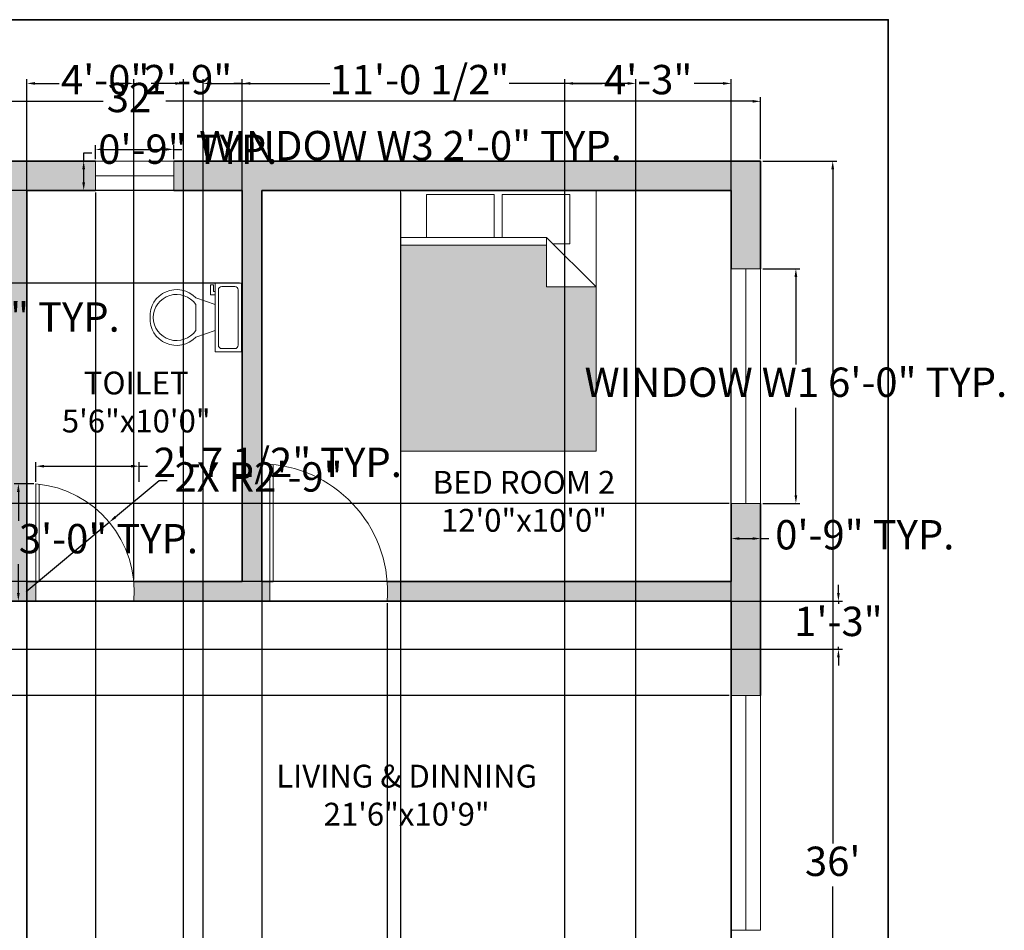
# Model space of a CAD drawing. Units: inches. Extents: x 2151 to 2709, y 3533 to 4046.
# Tile 4 of 4: x 2406 to 2708, y 3766 to 4046. Entities that reach past the tile are written whole.
import ezdxf

# ---------------------------------------------------------------- set-up
doc = ezdxf.new("R2010")
doc.units = ezdxf.units.IN
for name, color, linetype, lineweight in [('A-ANNO-DIMS', 2, 'Continuous', 18), ('A-ANNO-TTLB', 7, 'Continuous', 35), ('A-AREA-IDEN', 7, 'Continuous', 25), ('A-DOOR', 3, 'Continuous', 18), ('A-FLOR-FIXT', 8, 'Continuous', 18), ('A-FURN', 8, 'Continuous', 18), ('A-GLAZ', 4, 'Continuous', 18), ('A-WALL', 7, 'Continuous', 35)]:
    doc.layers.add(name, color=color, linetype=linetype, lineweight=lineweight)
doc.layers.add('A-FURN-PATT', color=107, linetype='Continuous', lineweight=13, true_color=0x477749)
doc.layers.add('A-WALL-PATT', color=18, linetype='Continuous', lineweight=13, true_color=0x000000)
doc.styles.get("Standard").update_dxf_attribs({"font": 'arial.ttf'})
doc.dimstyles.new('ISO-25', dxfattribs={"dimtxt": 9, "dimasz": 2.5, "dimexe": 1.25, "dimexo": 0.625, "dimgap": 2, "dimtad": 0, "dimtih": 1, "dimtoh": 1, "dimdec": 1, "dimlunit": 4, "dimtxsty": 'Standard', "dimcen": 2.5, "dimadec": 0, "dimazin": 0, "dimtfac": 0.5, "dimtdec": 1, "dimtmove": 0, "dimatfit": 3, "dimfxl": 1, "dimarcsym": 0})

# ---------------------------------------------------------------- blocks, each defined once
blk = doc.blocks.new('Bed - Queen')
for p, q in [((0, -80.00003), (0, 0)), ((0, 0), (59.99999, 0)), ((59.99999, 0), (59.99999, -80.00003)), ((7.99999, -1.2), (28.79998, -1.2)), ((7.99999, -14.4), (7.99999, -1.2)), ((28.79998, -1.2), (28.79998, -14.4)), ((31.19999, -1.2), (51.99999, -1.2)), ((31.19999, -14.4), (31.19999, -1.2)), ((51.99999, -1.2), (51.99999, -16.4)), ((0, -14.4), (44.8, -14.4)), ((59.99999, -29.6), (44.8, -14.4)), ((44.8, -14.4), (44.8, -29.6)), ((44.8, -16.8), (0, -16.8)), ((51.99999, -16.4), (46.79936, -16.4)), ((44.8, -29.6), (59.99999, -29.6)), ((59.99999, -80.00003), (0, -80.00003))]:
    blk.add_line(p, q)
blk = doc.blocks.new('*U3')
for p, q in [((9.5, -6), (9.5, -2)), ((-10, -8.5), (-8, -8.5)), ((-10, -9.5), (-10, -8.5)), ((-8, -8.5), (-8, -8)), ((-7, -8), (-7, -9.5)), ((-4, -8), (-6, -14)), ((4, -8), (6, -14)), ((-7, -9.5), (-10, -9.5)), ((4, -14), (-4, -14))]:
    blk.add_line(p, q)
blk.add_lwpolyline([(10.5, -8), (10.5, 0), (-10.5, 0), (-10.5, -8)], close=True)
for points in [[(-9.5, -2), (-9.5, -6)], [(8.5, -1), (-8.5, -1)], [(-8.5, -7), (8.5, -7)]]:
    blk.add_lwpolyline(points)
for centre, radius, start, end in [((-8.625, -1.875), 0.8839, 81.8699, 188.1301), ((8.625, -1.875), 0.8839, 351.8699, 98.1301), ((-8.625, -6.125), 0.8839, 171.869898, 278.1301), ((8.625, -6.125), 0.8839, 261.8699, 8.1301), ((-0.4772, -19.9188), 8.0953, 133.01722, 273.38), ((0.0374, -19.8731), 7.127, 124.50543, 269.7), ((-0.0373, -19.8731), 7.127, 270.3, 55.4946), ((0.4773, -19.9188), 8.0953, 266.62, 46.9828)]:
    blk.add_arc(centre, radius, start, end)
blk = doc.blocks.new('*D6')
at = {"layer": 'A-ANNO-DIMS', "color": 0, "lineweight": -2, "transparency": 16777216}
for p, q in [((2248.83, 4002.79), (2248.83, 4021.77)), ((2251.33, 4020.52), (2431.2, 4020.52)), ((2630.33, 4020.52), (2450.47, 4020.52)), ((2632.83, 4002.79), (2632.83, 4021.77))]:
    blk.add_line(p, q, dxfattribs=at)
at = {"layer": 'A-ANNO-DIMS', "color": 0, "transparency": 16777216}
for points in [[(2251.33, 4020.94), (2251.33, 4020.11), (2248.83, 4020.52)], [(2630.33, 4020.94), (2630.33, 4020.11), (2632.83, 4020.52)]]:
    blk.add_solid(points, dxfattribs=at)
at = {"layer": 'Defpoints', "color": 0, "transparency": 16777216}
for p in [(2632.83, 4020.52), (2248.83, 4002.17), (2632.83, 4002.17)]:
    blk.add_point(p, dxfattribs=at)
at = {"layer": 'A-ANNO-DIMS', "color": 0, "transparency": 16777216, "insert": (2440.83, 4020.52), "char_height": 9, "attachment_point": 5}
blk.add_mtext("32'", dxfattribs=at)
blk = doc.blocks.new('*D7')
at = {"layer": 'A-ANNO-DIMS', "color": 0, "lineweight": -2, "transparency": 16777216}
for p, q in [((2633.46, 4002.17), (2656.18, 4002.17)), ((2654.93, 3999.67), (2654.93, 3792.76)), ((2654.93, 3572.67), (2654.93, 3779.57)), ((2633.46, 3570.17), (2656.18, 3570.17))]:
    blk.add_line(p, q, dxfattribs=at)
at = {"layer": 'A-ANNO-DIMS', "color": 0, "transparency": 16777216}
for points in [[(2654.51, 3999.67), (2655.35, 3999.67), (2654.93, 4002.17)], [(2654.51, 3572.67), (2655.35, 3572.67), (2654.93, 3570.17)]]:
    blk.add_solid(points, dxfattribs=at)
at = {"layer": 'Defpoints', "color": 0, "transparency": 16777216}
for p in [(2632.83, 4002.17), (2632.83, 3570.17), (2654.93, 3570.17)]:
    blk.add_point(p, dxfattribs=at)
at = {"layer": 'A-ANNO-DIMS', "color": 0, "transparency": 16777216, "insert": (2654.93, 3786.17), "char_height": 9, "attachment_point": 5}
blk.add_mtext("36'", dxfattribs=at)
blk = doc.blocks.new('WIN-72IN')
for p, q in [((9, 72), (0, 72)), ((0, 72), (0, 0)), ((4.5, 0), (4.5, 72)), ((9, 72), (9, 0)), ((9, 0), (0, 0))]:
    blk.add_line(p, q)
blk = doc.blocks.new('WIN-24IN')
for p, q in [((0, 0), (0, 9)), ((0, 9), (24, 9)), ((24, 0), (24, 9)), ((0, 4.5), (24, 4.5)), ((0, 0), (24, 0))]:
    blk.add_line(p, q)
blk = doc.blocks.new('DOOR-SWING-36IN')
for p, q in [((0, 6), (0, 42)), ((1, 6), (1, 41.91)), ((0, 6), (0, 0)), ((0, 0), (36, 0))]:
    blk.add_line(p, q)
blk.add_arc((-3, 3), 39.12, 355.6013, 85.6013)
blk = doc.blocks.new('DOOR-SWING-30IN')
for p, q in [((0, 6), (0, 36)), ((1, 6), (1, 35.89)), ((0, 6), (0, 0)), ((0, 0), (30, 0))]:
    blk.add_line(p, q)
blk.add_arc((-3, 3), 33.14, 354.8056, 84.8056)
blk = doc.blocks.new('*D13')
at = {"layer": 'A-ANNO-DIMS', "color": 0, "lineweight": -2, "transparency": 16777216}
for p, q in [((2633.46, 3969.17), (2644.88, 3969.17)), ((2643.63, 3966.67), (2643.63, 3939.82)), ((2643.63, 3899.67), (2643.63, 3926.51)), ((2633.46, 3897.17), (2644.88, 3897.17))]:
    blk.add_line(p, q, dxfattribs=at)
at = {"layer": 'A-ANNO-DIMS', "color": 0, "transparency": 16777216}
for points in [[(2643.21, 3966.67), (2644.05, 3966.67), (2643.63, 3969.17)], [(2643.21, 3899.67), (2644.05, 3899.67), (2643.63, 3897.17)]]:
    blk.add_solid(points, dxfattribs=at)
at = {"layer": 'Defpoints', "color": 0, "transparency": 16777216}
for p in [(2632.83, 3969.17), (2643.63, 3969.17), (2632.83, 3897.17)]:
    blk.add_point(p, dxfattribs=at)
at = {"layer": 'A-ANNO-DIMS', "color": 0, "transparency": 16777216, "insert": (2643.63, 3933.17), "char_height": 9, "attachment_point": 5}
blk.add_mtext('WINDOW W1 6\'-0" TYP.', dxfattribs=at)
blk = doc.blocks.new('*D14')
at = {"layer": 'A-ANNO-DIMS', "color": 0, "lineweight": -2, "transparency": 16777216}
for p, q in [((2623.83, 3896.54), (2623.83, 3885.12)), ((2632.83, 3896.54), (2632.83, 3885.12)), ((2626.33, 3886.37), (2630.33, 3886.37)), ((2632.83, 3886.37), (2635.33, 3886.37))]:
    blk.add_line(p, q, dxfattribs=at)
at = {"layer": 'A-ANNO-DIMS', "color": 0, "transparency": 16777216}
for points in [[(2626.33, 3886.78), (2626.33, 3885.95), (2623.83, 3886.37)], [(2630.33, 3886.78), (2630.33, 3885.95), (2632.83, 3886.37)]]:
    blk.add_solid(points, dxfattribs=at)
at = {"layer": 'Defpoints', "color": 0, "transparency": 16777216}
for p in [(2623.83, 3897.17), (2632.83, 3897.17), (2632.83, 3886.37)]:
    blk.add_point(p, dxfattribs=at)
at = {"layer": 'A-ANNO-DIMS', "color": 0, "transparency": 16777216, "insert": (2664.76, 3886.37), "char_height": 9, "attachment_point": 5}
blk.add_mtext('0\'-9" TYP.', dxfattribs=at)
blk = doc.blocks.new('*D19')
at = {"layer": 'A-ANNO-DIMS', "color": 0, "lineweight": -2, "transparency": 16777216}
for p, q in [((2362.18, 3993.17), (2374.8, 3993.17)), ((2373.55, 3990.67), (2373.55, 3960.09)), ((2373.55, 3915.67), (2373.55, 3946.24)), ((2362.18, 3913.17), (2374.8, 3913.17))]:
    blk.add_line(p, q, dxfattribs=at)
at = {"layer": 'A-ANNO-DIMS', "color": 0, "transparency": 16777216}
for points in [[(2373.14, 3990.67), (2373.97, 3990.67), (2373.55, 3993.17)], [(2373.14, 3915.67), (2373.97, 3915.67), (2373.55, 3913.17)]]:
    blk.add_solid(points, dxfattribs=at)
at = {"layer": 'Defpoints', "color": 0, "transparency": 16777216}
for p in [(2361.55, 3993.17), (2373.55, 3993.17), (2361.55, 3913.17)]:
    blk.add_point(p, dxfattribs=at)
at = {"layer": 'A-ANNO-DIMS', "color": 0, "transparency": 16777216, "insert": (2373.55, 3953.17), "char_height": 9, "attachment_point": 5}
blk.add_mtext('QUEEN BED 6\'-8" TYP.', dxfattribs=at)
blk = doc.blocks.new('*D21')
at = {"layer": 'A-ANNO-DIMS', "color": 0, "lineweight": -2, "transparency": 16777216}
for p, q in [((2428.83, 4002.79), (2428.83, 4007.02)), ((2452.83, 4002.79), (2452.83, 4007.02)), ((2431.33, 4005.77), (2450.33, 4005.77)), ((2452.83, 4005.77), (2455.33, 4005.77))]:
    blk.add_line(p, q, dxfattribs=at)
at = {"layer": 'A-ANNO-DIMS', "color": 0, "transparency": 16777216}
for points in [[(2431.33, 4006.18), (2431.33, 4005.35), (2428.83, 4005.77)], [(2450.33, 4006.18), (2450.33, 4005.35), (2452.83, 4005.77)]]:
    blk.add_solid(points, dxfattribs=at)
at = {"layer": 'Defpoints', "color": 0, "transparency": 16777216}
for p in [(2452.83, 4005.77), (2428.83, 4002.17), (2452.83, 4002.17)]:
    blk.add_point(p, dxfattribs=at)
at = {"layer": 'A-ANNO-DIMS', "color": 0, "transparency": 16777216, "insert": (2525.45, 4005.77), "char_height": 9, "attachment_point": 5}
blk.add_mtext('WINDOW W3 2\'-0" TYP.', dxfattribs=at)
blk = doc.blocks.new('*D22')
at = {"layer": 'A-ANNO-DIMS', "color": 0, "lineweight": -2, "transparency": 16777216}
for p, q in [((2425.23, 4002.17), (2425.23, 4004.67)), ((2425.23, 4004.67), (2427.73, 4004.67)), ((2428.21, 4002.17), (2423.98, 4002.17)), ((2425.23, 3995.67), (2425.23, 3999.67)), ((2428.21, 3993.17), (2423.98, 3993.17))]:
    blk.add_line(p, q, dxfattribs=at)
at = {"layer": 'A-ANNO-DIMS', "color": 0, "transparency": 16777216}
for points in [[(2424.81, 3999.67), (2425.65, 3999.67), (2425.23, 4002.17)], [(2424.81, 3995.67), (2425.65, 3995.67), (2425.23, 3993.17)]]:
    blk.add_solid(points, dxfattribs=at)
at = {"layer": 'Defpoints', "color": 0, "transparency": 16777216}
for p in [(2425.23, 4002.17), (2428.83, 4002.17), (2428.83, 3993.17)]:
    blk.add_point(p, dxfattribs=at)
at = {"layer": 'A-ANNO-DIMS', "color": 0, "transparency": 16777216, "insert": (2457.16, 4004.67), "char_height": 9, "attachment_point": 5}
blk.add_mtext('0\'-9" TYP.', dxfattribs=at)
blk = doc.blocks.new('*D23')
at = {"layer": 'A-ANNO-DIMS', "color": 0, "lineweight": -2, "transparency": 16777216}
for p, q in [((2409.99, 3903.17), (2403.96, 3903.17)), ((2405.21, 3900.67), (2405.21, 3891.82)), ((2405.21, 3869.67), (2405.21, 3878.51)), ((2409.99, 3867.17), (2403.96, 3867.17))]:
    blk.add_line(p, q, dxfattribs=at)
at = {"layer": 'A-ANNO-DIMS', "color": 0, "transparency": 16777216}
for points in [[(2404.79, 3900.67), (2405.63, 3900.67), (2405.21, 3903.17)], [(2404.79, 3869.67), (2405.63, 3869.67), (2405.21, 3867.17)]]:
    blk.add_solid(points, dxfattribs=at)
at = {"layer": 'Defpoints', "color": 0, "transparency": 16777216}
for p in [(2405.21, 3903.17), (2410.61, 3903.17), (2410.61, 3867.17)]:
    blk.add_point(p, dxfattribs=at)
at = {"layer": 'A-ANNO-DIMS', "color": 0, "transparency": 16777216, "insert": (2405.21, 3885.17), "char_height": 9, "attachment_point": 5}
blk.add_mtext('DOOR D2 3\'-0" TYP.', dxfattribs=at)
blk = doc.blocks.new('*D24')
at = {"layer": 'A-ANNO-DIMS', "color": 0, "lineweight": -2, "transparency": 16777216}
for p, q in [((2410.61, 3903.79), (2410.61, 3909.82)), ((2413.11, 3908.57), (2439.77, 3908.57)), ((2442.27, 3903.79), (2442.27, 3909.82)), ((2442.27, 3908.57), (2444.77, 3908.57))]:
    blk.add_line(p, q, dxfattribs=at)
at = {"layer": 'A-ANNO-DIMS', "color": 0, "transparency": 16777216}
for points in [[(2413.11, 3908.98), (2413.11, 3908.15), (2410.61, 3908.57)], [(2439.77, 3908.98), (2439.77, 3908.15), (2442.27, 3908.57)]]:
    blk.add_solid(points, dxfattribs=at)
at = {"layer": 'Defpoints', "color": 0, "transparency": 16777216}
for p in [(2442.27, 3908.57), (2410.61, 3903.17), (2442.27, 3903.17)]:
    blk.add_point(p, dxfattribs=at)
at = {"layer": 'A-ANNO-DIMS', "color": 0, "transparency": 16777216, "insert": (2484.76, 3908.57), "char_height": 9, "attachment_point": 5}
blk.add_mtext('2\'-7 1/2" TYP.', dxfattribs=at)
blk = doc.blocks.new('*D25')
at = {"layer": 'A-ANNO-DIMS', "color": 0, "lineweight": -2, "transparency": 16777216}
for p, q in [((2407.83, 3737.79), (2407.83, 4027.27)), ((2410.33, 4026.02), (2417.69, 4026.02)), ((2453.33, 4026.02), (2445.97, 4026.02)), ((2455.83, 3737.79), (2455.83, 4027.27))]:
    blk.add_line(p, q, dxfattribs=at)
at = {"layer": 'A-ANNO-DIMS', "color": 0, "transparency": 16777216}
for points in [[(2410.33, 4026.43), (2410.33, 4025.6), (2407.83, 4026.02)], [(2453.33, 4026.43), (2453.33, 4025.6), (2455.83, 4026.02)]]:
    blk.add_solid(points, dxfattribs=at)
at = {"layer": 'Defpoints', "color": 0, "transparency": 16777216}
for p in [(2455.83, 4026.02), (2407.83, 3737.17), (2455.83, 3737.17)]:
    blk.add_point(p, dxfattribs=at)
at = {"layer": 'A-ANNO-DIMS', "color": 0, "transparency": 16777216, "insert": (2431.83, 4026.02), "char_height": 9, "attachment_point": 5}
blk.add_mtext('4\'-0"', dxfattribs=at)
blk = doc.blocks.new('*D30')
at = {"layer": 'A-ANNO-DIMS', "color": 0, "lineweight": -2, "transparency": 16777216}
for p, q in [((2623.21, 3867.17), (2173.29, 3867.17)), ((2174.54, 3864.67), (2174.54, 3859.26)), ((2174.54, 3840.67), (2174.54, 3846.07)), ((2623.21, 3838.17), (2173.29, 3838.17))]:
    blk.add_line(p, q, dxfattribs=at)
at = {"layer": 'A-ANNO-DIMS', "color": 0, "transparency": 16777216}
for points in [[(2174.13, 3864.67), (2174.96, 3864.67), (2174.54, 3867.17)], [(2174.13, 3840.67), (2174.96, 3840.67), (2174.54, 3838.17)]]:
    blk.add_solid(points, dxfattribs=at)
at = {"layer": 'Defpoints', "color": 0, "transparency": 16777216}
for p in [(2174.54, 3867.17), (2623.83, 3867.17), (2623.83, 3838.17)]:
    blk.add_point(p, dxfattribs=at)
at = {"layer": 'A-ANNO-DIMS', "color": 0, "transparency": 16777216, "insert": (2174.54, 3852.67), "char_height": 9, "attachment_point": 5}
blk.add_mtext('2\'-5"', dxfattribs=at)
blk = doc.blocks.new('*D31')
at = {"layer": 'A-ANNO-DIMS', "color": 0, "lineweight": -2, "transparency": 16777216}
for p, q in [((2623.21, 3897.17), (2173.29, 3897.17)), ((2174.54, 3894.67), (2174.54, 3891.76)), ((2174.54, 3875.67), (2174.54, 3878.57)), ((2623.21, 3873.17), (2173.29, 3873.17))]:
    blk.add_line(p, q, dxfattribs=at)
at = {"layer": 'A-ANNO-DIMS', "color": 0, "transparency": 16777216}
for points in [[(2174.13, 3894.67), (2174.96, 3894.67), (2174.54, 3897.17)], [(2174.13, 3875.67), (2174.96, 3875.67), (2174.54, 3873.17)]]:
    blk.add_solid(points, dxfattribs=at)
at = {"layer": 'Defpoints', "color": 0, "transparency": 16777216}
for p in [(2174.54, 3897.17), (2623.83, 3897.17), (2623.83, 3873.17)]:
    blk.add_point(p, dxfattribs=at)
at = {"layer": 'A-ANNO-DIMS', "color": 0, "transparency": 16777216, "insert": (2174.54, 3885.17), "char_height": 9, "attachment_point": 5}
blk.add_mtext('2\'-0"', dxfattribs=at)
blk = doc.blocks.new('*D34')
at = {"layer": 'A-ANNO-DIMS', "color": 0, "lineweight": -2, "transparency": 16777216}
for p, q in [((2572.83, 3643.79), (2572.83, 4027.27)), ((2575.33, 4026.02), (2584.19, 4026.02)), ((2621.33, 4026.02), (2612.47, 4026.02)), ((2623.83, 3643.79), (2623.83, 4027.27))]:
    blk.add_line(p, q, dxfattribs=at)
at = {"layer": 'A-ANNO-DIMS', "color": 0, "transparency": 16777216}
for points in [[(2575.33, 4026.43), (2575.33, 4025.6), (2572.83, 4026.02)], [(2621.33, 4026.43), (2621.33, 4025.6), (2623.83, 4026.02)]]:
    blk.add_solid(points, dxfattribs=at)
at = {"layer": 'Defpoints', "color": 0, "transparency": 16777216}
for p in [(2623.83, 4026.02), (2572.83, 3643.17), (2623.83, 3643.17)]:
    blk.add_point(p, dxfattribs=at)
at = {"layer": 'A-ANNO-DIMS', "color": 0, "transparency": 16777216, "insert": (2598.33, 4026.02), "char_height": 9, "attachment_point": 5}
blk.add_mtext('4\'-3"', dxfattribs=at)
blk = doc.blocks.new('*D39')
at = {"layer": 'A-ANNO-DIMS', "color": 0, "lineweight": -2, "transparency": 16777216}
for p, q in [((2407.83, 3992.54), (2407.83, 3545.07)), ((2428.83, 3992.54), (2428.83, 3545.07)), ((2410.33, 3546.32), (2426.33, 3546.32)), ((2428.83, 3546.32), (2431.33, 3546.32))]:
    blk.add_line(p, q, dxfattribs=at)
at = {"layer": 'A-ANNO-DIMS', "color": 0, "transparency": 16777216}
for points in [[(2410.33, 3546.73), (2410.33, 3545.9), (2407.83, 3546.32)], [(2426.33, 3546.73), (2426.33, 3545.9), (2428.83, 3546.32)]]:
    blk.add_solid(points, dxfattribs=at)
at = {"layer": 'Defpoints', "color": 0, "transparency": 16777216}
for p in [(2407.83, 3993.17), (2428.83, 3993.17), (2428.83, 3546.32)]:
    blk.add_point(p, dxfattribs=at)
at = {"layer": 'A-ANNO-DIMS', "color": 0, "transparency": 16777216, "insert": (2444.87, 3546.32), "char_height": 9, "attachment_point": 5}
blk.add_mtext('1\'-9"', dxfattribs=at)
blk = doc.blocks.new('*D42')
at = {"layer": 'A-ANNO-DIMS', "color": 0, "lineweight": -2, "transparency": 16777216}
for p, q in [((2479.83, 3992.54), (2479.83, 3545.07)), ((2522.34, 3992.54), (2522.34, 3545.07)), ((2479.83, 3546.32), (2477.33, 3546.32)), ((2519.84, 3546.32), (2482.33, 3546.32))]:
    blk.add_line(p, q, dxfattribs=at)
at = {"layer": 'A-ANNO-DIMS', "color": 0, "transparency": 16777216}
for points in [[(2482.33, 3546.73), (2482.33, 3545.9), (2479.83, 3546.32)], [(2519.84, 3546.73), (2519.84, 3545.9), (2522.34, 3546.32)]]:
    blk.add_solid(points, dxfattribs=at)
at = {"layer": 'Defpoints', "color": 0, "transparency": 16777216}
for p in [(2479.83, 3993.17), (2522.34, 3993.17), (2479.83, 3546.32)]:
    blk.add_point(p, dxfattribs=at)
at = {"layer": 'A-ANNO-DIMS', "color": 0, "transparency": 16777216, "insert": (2452.89, 3546.32), "char_height": 9, "attachment_point": 5}
blk.add_mtext('3\'-6 1/2"', dxfattribs=at)
blk = doc.blocks.new('*D43')
at = {"layer": 'A-ANNO-DIMS', "color": 0, "lineweight": -2, "transparency": 16777216}
for p, q in [((2461.83, 3737.79), (2461.83, 4027.27)), ((2464.33, 4026.02), (2500.67, 4026.02)), ((2592.05, 4026.02), (2555.71, 4026.02)), ((2594.55, 3737.79), (2594.55, 4027.27))]:
    blk.add_line(p, q, dxfattribs=at)
at = {"layer": 'A-ANNO-DIMS', "color": 0, "transparency": 16777216}
for points in [[(2464.33, 4026.43), (2464.33, 4025.6), (2461.83, 4026.02)], [(2592.05, 4026.43), (2592.05, 4025.6), (2594.55, 4026.02)]]:
    blk.add_solid(points, dxfattribs=at)
at = {"layer": 'Defpoints', "color": 0, "transparency": 16777216}
for p in [(2594.55, 4026.02), (2461.83, 3737.17), (2594.55, 3737.17)]:
    blk.add_point(p, dxfattribs=at)
at = {"layer": 'A-ANNO-DIMS', "color": 0, "transparency": 16777216, "insert": (2528.19, 4026.02), "char_height": 9, "attachment_point": 5}
blk.add_mtext('11\'-0 1/2"', dxfattribs=at)
blk = doc.blocks.new('*D47')
at = {"layer": 'A-ANNO-DIMS', "color": 0, "lineweight": -2, "transparency": 16777216}
for p, q in [((2518.29, 3866.54), (2518.29, 3545.07)), ((2623.83, 3866.54), (2623.83, 3545.07)), ((2520.79, 3546.32), (2546.61, 3546.32)), ((2621.33, 3546.32), (2595.52, 3546.32))]:
    blk.add_line(p, q, dxfattribs=at)
at = {"layer": 'A-ANNO-DIMS', "color": 0, "transparency": 16777216}
for points in [[(2520.79, 3546.73), (2520.79, 3545.9), (2518.29, 3546.32)], [(2621.33, 3546.73), (2621.33, 3545.9), (2623.83, 3546.32)]]:
    blk.add_solid(points, dxfattribs=at)
at = {"layer": 'Defpoints', "color": 0, "transparency": 16777216}
for p in [(2518.29, 3867.17), (2623.83, 3867.17), (2623.83, 3546.32)]:
    blk.add_point(p, dxfattribs=at)
at = {"layer": 'A-ANNO-DIMS', "color": 0, "transparency": 16777216, "insert": (2571.06, 3546.32), "char_height": 9, "attachment_point": 5}
blk.add_mtext('8\'-9 1/2"', dxfattribs=at)
blk = doc.blocks.new('*D52')
at = {"layer": 'A-ANNO-DIMS', "color": 0, "lineweight": -2, "transparency": 16777216}
for p, q in [((2473.21, 3993.17), (2173.29, 3993.17)), ((2174.54, 3990.67), (2174.54, 3985.58)), ((2174.54, 3967.19), (2174.54, 3972.27)), ((2472.97, 3964.69), (2173.29, 3964.69))]:
    blk.add_line(p, q, dxfattribs=at)
at = {"layer": 'A-ANNO-DIMS', "color": 0, "transparency": 16777216}
for points in [[(2174.13, 3990.67), (2174.96, 3990.67), (2174.54, 3993.17)], [(2174.13, 3967.19), (2174.96, 3967.19), (2174.54, 3964.69)]]:
    blk.add_solid(points, dxfattribs=at)
at = {"layer": 'Defpoints', "color": 0, "transparency": 16777216}
for p in [(2473.83, 3993.17), (2174.54, 3964.69), (2473.59, 3964.69)]:
    blk.add_point(p, dxfattribs=at)
at = {"layer": 'A-ANNO-DIMS', "color": 0, "transparency": 16777216, "insert": (2174.54, 3978.93), "char_height": 9, "attachment_point": 5}
blk.add_mtext('2\'-4 1/2"', dxfattribs=at)
blk = doc.blocks.new('*D53')
at = {"layer": 'A-ANNO-DIMS', "color": 0, "lineweight": -2, "transparency": 16777216}
for p, q in [((2656.68, 3869.67), (2656.68, 3872.17)), ((2258.46, 3867.17), (2657.93, 3867.17)), ((2656.68, 3867.17), (2656.68, 3866.37)), ((2656.68, 3852.39), (2656.68, 3853.18)), ((2259.02, 3852.39), (2657.93, 3852.39)), ((2656.68, 3849.89), (2656.68, 3847.39))]:
    blk.add_line(p, q, dxfattribs=at)
at = {"layer": 'A-ANNO-DIMS', "color": 0, "transparency": 16777216}
for points in [[(2656.26, 3869.67), (2657.1, 3869.67), (2656.68, 3867.17)], [(2656.26, 3849.89), (2657.1, 3849.89), (2656.68, 3852.39)]]:
    blk.add_solid(points, dxfattribs=at)
at = {"layer": 'Defpoints', "color": 0, "transparency": 16777216}
for p in [(2257.83, 3867.17), (2656.68, 3867.17), (2258.39, 3852.39)]:
    blk.add_point(p, dxfattribs=at)
at = {"layer": 'A-ANNO-DIMS', "color": 0, "transparency": 16777216, "insert": (2656.68, 3859.78), "char_height": 9, "attachment_point": 5}
blk.add_mtext('1\'-3"', dxfattribs=at)
blk = doc.blocks.new('*D54')
at = {"layer": 'A-ANNO-DIMS', "color": 0, "lineweight": -2, "transparency": 16777216}
for p, q in [((2438.11, 4026.02), (2435.61, 4026.02)), ((2440.61, 3873.79), (2440.61, 4027.27)), ((2440.61, 4026.02), (2443.18, 4026.02)), ((2473.83, 4026.02), (2471.26, 4026.02)), ((2473.83, 3873.79), (2473.83, 4027.27)), ((2476.33, 4026.02), (2478.83, 4026.02))]:
    blk.add_line(p, q, dxfattribs=at)
at = {"layer": 'A-ANNO-DIMS', "color": 0, "transparency": 16777216}
for points in [[(2438.11, 4026.43), (2438.11, 4025.6), (2440.61, 4026.02)], [(2476.33, 4026.43), (2476.33, 4025.6), (2473.83, 4026.02)]]:
    blk.add_solid(points, dxfattribs=at)
at = {"layer": 'Defpoints', "color": 0, "transparency": 16777216}
for p in [(2473.83, 4026.02), (2440.61, 3873.17), (2473.83, 3873.17)]:
    blk.add_point(p, dxfattribs=at)
at = {"layer": 'A-ANNO-DIMS', "color": 0, "transparency": 16777216, "insert": (2457.22, 4026.02), "char_height": 9, "attachment_point": 5}
blk.add_mtext('2\'-9"', dxfattribs=at)
blk = doc.blocks.new('*D58')
at = {"layer": 'A-ANNO-DIMS', "color": 0, "lineweight": -2, "transparency": 16777216}
for p, q in [((2448.34, 3904.11), (2434.99, 3892.98)), ((2450.84, 3904.11), (2448.34, 3904.11)), ((2407.61, 3870.17), (2433.07, 3891.38))]:
    blk.add_line(p, q, dxfattribs=at)
at = {"layer": 'A-ANNO-DIMS', "color": 0, "transparency": 16777216}
blk.add_solid([(2434.72, 3893.3), (2435.25, 3892.66), (2433.07, 3891.38)], dxfattribs=at)
at = {"layer": 'Defpoints', "color": 0, "transparency": 16777216}
for p in [(2433.07, 3891.38), (2407.61, 3870.17)]:
    blk.add_point(p, dxfattribs=at)
at = {"layer": 'A-ANNO-DIMS', "color": 0, "transparency": 16777216, "insert": (2478.85, 3904.11), "char_height": 9, "attachment_point": 5}
blk.add_mtext('2X R2\'-9"', dxfattribs=at)

msp = doc.modelspace()

# ---------------------------------------------------------------- hatches: boundary and pattern name
at = {"layer": 'A-FURN-PATT'}
h = msp.add_hatch(color=256, dxfattribs=at)
h.dxf.hatch_style = 1
h.paths.add_polyline_path([(2361.55, 3963.57), (2346.35, 3963.57), (2346.35, 3976.37), (2301.55, 3976.37), (2301.55, 3913.17), (2361.55, 3913.17)])
h.paths.add_polyline_path([(2582.34, 3963.57), (2567.14, 3963.57), (2567.14, 3976.37), (2522.34, 3976.37), (2522.34, 3913.17), (2582.34, 3913.17)])
at = {"layer": 'A-WALL-PATT'}
h = msp.add_hatch(color=256, dxfattribs=at)
h.dxf.hatch_style = 1
h.paths.add_polyline_path([(2428.83, 4002.17), (2248.83, 4002.17), (2248.83, 3969.17), (2257.83, 3969.17), (2257.83, 3993.16), (2401.83, 3993.16), (2401.83, 3873.17), (2399.81, 3873.17), (2399.81, 3867.16), (2410.61, 3867.16), (2410.61, 3873.17), (2407.83, 3873.17), (2407.83, 3993.16), (2428.83, 3993.16)])
h.paths.add_polyline_path([(2632.83, 4002.17), (2452.83, 4002.17), (2452.83, 3993.16), (2473.83, 3993.16), (2473.83, 3873.17), (2440.61, 3873.17, -0.045361), (2440.61, 3867.16), (2482.29, 3867.16), (2482.29, 3873.17), (2479.83, 3873.17), (2479.83, 3993.16), (2623.83, 3993.16), (2623.83, 3969.17), (2632.83, 3969.17)])
h.paths.add_polyline_path([(2257.83, 3897.17), (2248.83, 3897.17), (2248.83, 3853.17), (2257.83, 3853.17), (2257.83, 3867.16), (2324.99, 3867.16, -0.045361), (2324.99, 3873.17), (2257.83, 3873.17)])
h.paths.add_polyline_path([(2632.83, 3897.17), (2623.83, 3897.17), (2623.83, 3873.17), (2518.29, 3873.17, -0.038405), (2518.29, 3867.16), (2623.83, 3867.16), (2623.83, 3838.17), (2632.83, 3838.17)])
h.paths.add_polyline_path([(2364.83, 3815.17), (2364.83, 3867.16), (2365.88, 3867.16, -0.038164), (2365.88, 3873.17), (2354.99, 3873.17), (2354.99, 3867.16), (2358.83, 3867.16), (2358.83, 3815.17), (2257.83, 3815.17), (2257.83, 3829.17), (2248.83, 3829.17), (2248.83, 3797.17), (2257.83, 3797.17), (2257.83, 3809.17), (2358.83, 3809.17), (2364.83, 3809.17)])
h.paths.add_polyline_path([(2364.21, 3737.17), (2257.83, 3737.17), (2257.83, 3749.17), (2248.83, 3749.17), (2248.83, 3685.17), (2257.83, 3685.17), (2257.83, 3731.17), (2364.21, 3731.17, -0.038405)])
h.paths.add_polyline_path([(2257.83, 3625.17), (2248.83, 3625.17), (2248.83, 3570.17), (2299.83, 3570.17), (2299.83, 3579.17), (2257.83, 3579.17)])

# ---------------------------------------------------------------- linework, layer by layer
at = {"layer": 'A-ANNO-TTLB'}
msp.add_lwpolyline([(2228.43, 4045.57), (2671.96, 4045.57), (2671.96, 3550.81), (2228.43, 3550.81)], close=True, dxfattribs=at)
at = {"layer": 'A-WALL'}
for p, q in [((2248.83, 4002.17), (2428.83, 4002.17)), ((2452.83, 4002.17), (2632.83, 4002.17)), ((2632.83, 4002.17), (2632.83, 3969.17)), ((2407.83, 3873.17), (2407.83, 3993.16)), ((2407.83, 3993.16), (2428.83, 3993.16)), ((2407.83, 3993.16), (2428.83, 3993.16)), ((2452.83, 3993.16), (2473.83, 3993.16)), ((2452.83, 3993.16), (2473.83, 3993.16)), ((2473.83, 3873.17), (2473.83, 3993.16)), ((2479.83, 3873.17), (2479.83, 3993.16)), ((2479.83, 3993.16), (2623.83, 3993.16)), ((2479.83, 3993.16), (2623.83, 3993.16)), ((2623.83, 3993.16), (2623.83, 3969.17)), ((2623.83, 3897.17), (2623.83, 3873.17)), ((2632.83, 3897.17), (2632.83, 3838.17)), ((2407.83, 3873.17), (2411.61, 3873.17)), ((2440.61, 3873.17), (2473.83, 3873.17)), ((2479.83, 3873.17), (2483.29, 3873.17)), ((2518.29, 3873.17), (2623.83, 3873.17)), ((2399.81, 3867.16), (2410.61, 3867.16)), ((2440.61, 3867.16), (2482.29, 3867.16)), ((2518.29, 3867.16), (2623.83, 3867.16)), ((2623.83, 3867.16), (2623.83, 3838.17))]:
    msp.add_line(p, q, dxfattribs=at)

# ---------------------------------------------------------------- block references
at = {"layer": 'A-DOOR'}
for name, p in [('DOOR-SWING-36IN', (2482.29, 3867.16)), ('DOOR-SWING-30IN', (2410.61, 3867.16))]:
    msp.add_blockref(name, p, dxfattribs=at)
at = {"layer": 'A-FLOR-FIXT', "rotation": 270}
msp.add_blockref('*U3', (2473.59, 3954.19), dxfattribs=at)
at = {"layer": 'A-FURN'}
msp.add_blockref('Bed - Queen', (2522.34, 3993.16), dxfattribs=at)
at = {"layer": 'A-GLAZ'}
for name, p in [('WIN-24IN', (2428.83, 3993.16)), ('WIN-72IN', (2623.83, 3897.17)), ('WIN-72IN', (2623.83, 3766.17))]:
    msp.add_blockref(name, p, dxfattribs=at)

# ---------------------------------------------------------------- texts
at = {"layer": 'A-AREA-IDEN', "char_height": 7, "attachment_point": 1}
for s, width, insert in [('\\pxqc;{\\fArial|b1|i0|c0|p34;TOILET\\P5\'6"x10\'0"}', 56.7116, (2412.98, 3937.59)), ('\\pxqc;{\\fArial|b1|i0|c0|p34;BED ROOM 2\\P12\'0"x10\'0"}', 63.7068, (2528.4, 3907.13)), ('\\pxqc;{\\fArial|b1|i0|c0|p34;LIVING & DINNING\\P21\'6"x10\'9"}', 116.9296, (2465.81, 3816.97))]:
    msp.add_mtext_dynamic_manual_height_columns(s, width=width, gutter_width=12.5, heights=[0], dxfattribs=dict(at, insert=insert))

# ---------------------------------------------------------------- dimensions: what is measured, and where the dimension line sits
at = {"layer": 'A-ANNO-DIMS'}
for base, p1, p2, override, picture, middle in [((2594.55, 4026.02), (2461.83, 3737.17), (2594.55, 3737.17), {"dimdec": 1, "dimlfac": 1, "dimrnd": 0, "dimzin": 1, "dimdsep": 46, "dimlunit": 4, "dimfrac": 2}, '*D43', (2528.19, 4026.02)), ((2455.83, 4026.02), (2407.83, 3737.17), (2455.83, 3737.17), {"dimdec": 1, "dimlfac": 1, "dimrnd": 0, "dimzin": 1, "dimdsep": 46, "dimlunit": 4, "dimfrac": 2}, '*D25', (2431.83, 4026.02)), ((2473.83, 4026.02), (2440.61, 3873.17), (2473.83, 3873.17), {"dimdec": 1, "dimlfac": 1, "dimrnd": 0, "dimzin": 1, "dimdsep": 46, "dimlunit": 4, "dimfrac": 2}, '*D54', (2457.22, 4026.02)), ((2623.83, 4026.02), (2572.83, 3643.17), (2623.83, 3643.17), {"dimdec": 1, "dimlfac": 1, "dimrnd": 0, "dimzin": 1, "dimdsep": 46, "dimlunit": 4, "dimfrac": 2}, '*D34', (2598.33, 4026.02)), ((2632.83, 4020.52), (2248.83, 4002.17), (2632.83, 4002.17), {"dimclrd": 0, "dimclre": 0, "dimclrt": 0}, '*D6', (2440.83, 4020.52)), ((2428.83, 3546.32), (2407.83, 3993.16), (2428.83, 3993.16), {"dimdec": 1, "dimlfac": 1, "dimrnd": 0, "dimzin": 1, "dimdsep": 46, "dimlunit": 4, "dimfrac": 2}, '*D39', (2444.87, 3546.32)), ((2479.83, 3546.32), (2522.34, 3993.16), (2479.83, 3993.16), {"dimdec": 1, "dimlfac": 1, "dimrnd": 0, "dimzin": 1, "dimdsep": 46, "dimlunit": 4, "dimfrac": 2}, '*D42', (2452.89, 3546.32)), ((2623.83, 3546.32), (2518.29, 3867.16), (2623.83, 3867.16), {"dimdec": 1, "dimlfac": 1, "dimrnd": 0, "dimzin": 1, "dimdsep": 46, "dimlunit": 4, "dimfrac": 2}, '*D47', (2571.06, 3546.32))]:
    dim = msp.add_linear_dim(base=base, p1=p1, p2=p2, dimstyle='ISO-25', override=override, dxfattribs=at)
    dim.commit()
    dim.dimension.update_dxf_attribs({"geometry": picture, "text_midpoint": middle})
for base, p1, p2, text, picture, middle in [((2452.83, 4005.77), (2428.83, 4002.17), (2452.83, 4002.17), 'WINDOW W3 <> TYP.', '*D21', (2525.45, 4005.77)), ((2442.27, 3908.57), (2410.61, 3903.17), (2442.27, 3903.17), '<> TYP.', '*D24', (2484.76, 3908.57)), ((2632.83, 3886.37), (2623.83, 3897.17), (2632.83, 3897.17), '<> TYP.', '*D14', (2664.76, 3886.37))]:
    dim = msp.add_linear_dim(base=base, p1=p1, p2=p2, text=text, dimstyle='ISO-25', override={"dimdec": 1, "dimlfac": 1, "dimrnd": 0, "dimzin": 1, "dimdsep": 46, "dimlunit": 4, "dimfrac": 2}, dxfattribs=at)
    dim.commit()
    dim.dimension.update_dxf_attribs({"geometry": picture, "text_midpoint": middle})
for base, p1, p2, text, picture, middle in [((2425.23, 4002.17), (2428.83, 3993.16), (2428.83, 4002.17), '<> TYP.', '*D22', (2457.16, 4004.67)), ((2373.55, 3993.16), (2361.55, 3913.17), (2361.55, 3993.16), 'QUEEN BED <> TYP.', '*D19', (2373.55, 3953.17)), ((2643.63, 3969.17), (2632.83, 3897.17), (2632.83, 3969.17), 'WINDOW W1 <> TYP.', '*D13', (2643.63, 3933.17)), ((2405.21, 3903.17), (2410.61, 3867.16), (2410.61, 3903.17), 'DOOR D2 <> TYP.', '*D23', (2405.21, 3885.17))]:
    dim = msp.add_linear_dim(base=base, p1=p1, p2=p2, angle=90, text=text, dimstyle='ISO-25', override={"dimdec": 1, "dimlfac": 1, "dimrnd": 0, "dimzin": 1, "dimdsep": 46, "dimlunit": 4, "dimfrac": 2}, dxfattribs=at)
    dim.commit()
    dim.dimension.update_dxf_attribs({"geometry": picture, "text_midpoint": middle})
for base, p1, p2, override, picture, middle in [((2654.93, 3570.17), (2632.83, 4002.17), (2632.83, 3570.17), {"dimclrd": 0, "dimclre": 0, "dimclrt": 0}, '*D7', (2654.93, 3786.17)), ((2174.54, 3964.69), (2473.83, 3993.16), (2473.59, 3964.69), {"dimdec": 1, "dimlfac": 1, "dimrnd": 0, "dimzin": 1, "dimdsep": 46, "dimlunit": 4, "dimfrac": 2}, '*D52', (2174.54, 3978.93)), ((2174.54, 3897.17), (2623.83, 3873.17), (2623.83, 3897.17), {"dimdec": 1, "dimlfac": 1, "dimrnd": 0, "dimzin": 1, "dimdsep": 46, "dimlunit": 4, "dimfrac": 2}, '*D31', (2174.54, 3885.17)), ((2656.68, 3867.16), (2258.39, 3852.39), (2257.83, 3867.16), {"dimdec": 1, "dimlfac": 1, "dimrnd": 0, "dimzin": 1, "dimdsep": 46, "dimlunit": 4, "dimfrac": 2}, '*D53', (2656.68, 3859.78)), ((2174.54, 3867.16), (2623.83, 3838.17), (2623.83, 3867.16), {"dimdec": 1, "dimlfac": 1, "dimrnd": 0, "dimzin": 1, "dimdsep": 46, "dimlunit": 4, "dimfrac": 2}, '*D30', (2174.54, 3852.67))]:
    dim = msp.add_linear_dim(base=base, p1=p1, p2=p2, angle=90, dimstyle='ISO-25', override=override, dxfattribs=at)
    dim.commit()
    dim.dimension.update_dxf_attribs({"geometry": picture, "text_midpoint": middle})
dim = msp.add_radius_dim(center=(2407.61, 3870.17), mpoint=(2433.07, 3891.38), text='2X <>', dimstyle='ISO-25', override={"dimdec": 1, "dimlfac": 1, "dimrnd": 0, "dimzin": 1, "dimdsep": 46, "dimlunit": 4, "dimfrac": 2}, dxfattribs=at)
dim.commit()
dim.dimension.update_dxf_attribs({"geometry": '*D58', "text_midpoint": (2478.85, 3904.11), "dimtype": 164})

doc.saveas('drawing.dxf')
